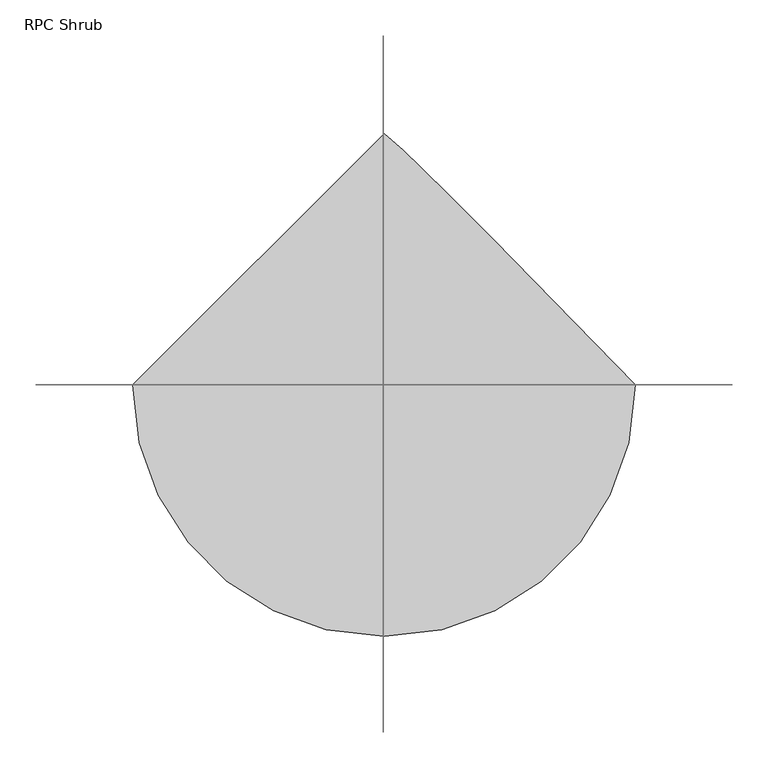
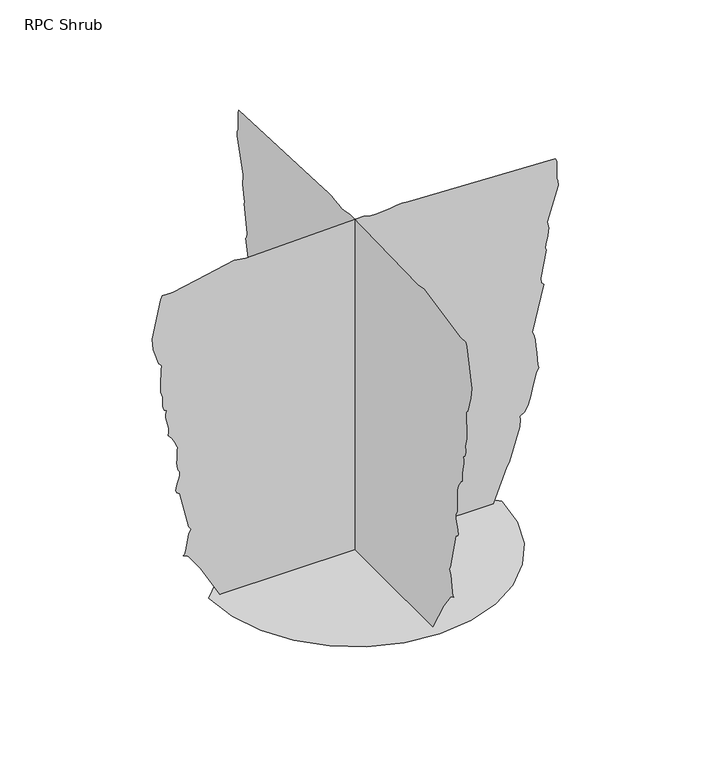
"""IFC4 building model written with IfcOpenShell, lengths in millimetres: geographic element geometry, RPC Shrub."""

from ifc_helpers import new_model, si_unit, origin, place, context, project, spatial, triangles, source, transform, mapped, element, save


def rpc_shrub_31a8b93a(model_context):
    return source(origin(), model_context, "Body", "Tessellation", [
        triangles([(-350.7919238, 0.0, 0.0), (-341.5167269, -80.3781425, 0.0), (-315.1055846, -154.1926595, 0.0), (-273.6723033, -219.3286546, 0.0), (-219.3286546, -273.6723033, 0.0), (-154.1926595, -315.1055846, 0.0), (-80.3781425, -341.5167269, 0.0), (1.53e-05, -350.7919238, 0.0), (80.3781425, -341.5167269, 0.0), (154.1926595, -315.1055846, 0.0), (219.3286546, -273.6723033, 0.0), (273.6723033, -219.3286546, 0.0), (315.1055846, -154.1926595, 0.0), (341.5167269, -80.3781425, 0.0), (350.7919238, 3.07e-05, 0.0), (236.7920327, 116.9354496, 0.0), (152.278414, 203.0298493, 0.0), (92.3366331, 263.4226928, 0.0), (52.0522189, 303.2555267, 0.0), (26.5109567, 327.6680809, 0.0), (10.7982689, 341.7996311, 0.0), (-4.6e-05, 350.7919238, 0.0), (-324.215748, 3.84e-05, 1.2173179), (-370.8406274, 3.35e-05, 83.4658628), (-399.9261703, 3.11e-05, 123.0734289), (-412.2293801, 3.08e-05, 129.051625), (-408.9211155, 3.06e-05, 131.6657641), (-406.1157635, 3.01e-05, 140.3154633), (-403.6090124, 2.93e-05, 152.586453), (-401.2018192, 2.85e-05, 166.0644457), (-398.6976843, 2.78e-05, 178.3356989), (-395.8897161, 2.73e-05, 186.9853889), (-392.5840676, 2.72e-05, 189.5995281), (-398.4933726, 2.67e-05, 197.4594953), (-420.6166225, 2.13e-05, 288.7310862), (-428.0425501, 2.09e-05, 294.8263719), (-430.4602441, 2.06e-05, 300.2222816), (-429.3784424, 2.01e-05, 307.9153985), (-426.2954184, 1.96e-05, 317.0255619), (-422.7147503, 1.9e-05, 326.6727201), (-420.1294066, 1.84e-05, 335.9714985), (-420.0429657, 1.8e-05, 344.0470593), (-423.9458525, 1.76e-05, 350.0113755), (-425.7846574, 1.73e-05, 354.1133054), (-426.7642851, 1.69e-05, 361.0677501), (-427.0864675, 1.64e-05, 370.0050679), (-426.9502839, 1.58e-05, 380.0529648), (-426.549509, 1.52e-05, 390.3444878), (-426.0858745, 1.46e-05, 400.0073791), (-425.7532276, 1.41e-05, 408.1745768), (-426.4709164, 1.4e-05, 410.2203094), (-428.5533111, 1.37e-05, 415.1395223), (-431.6808455, 1.33e-05, 421.8555731), (-435.5339533, 1.29e-05, 429.2946176), (-439.7930683, 1.24e-05, 436.3773974), (-444.1438565, 1.21e-05, 442.0247635), (-448.2641356, 1.19e-05, 445.1627987), (-446.5798634, 1.13e-05, 454.7627941), (-447.3237496, 1.08e-05, 464.614264), (-449.4533072, 1.02e-05, 474.4814306), (-451.9312446, 9.6e-06, 484.1285889), (-453.7228867, 9.1e-06, 493.3199973), (-453.7857462, 8.6e-06, 501.8172257), (-451.0825682, 8.1e-06, 509.3872215), (-457.0521166, 7.8e-06, 513.5415828), (-460.0617803, 7.5e-06, 518.8850793), (-461.0545249, 7.1e-06, 525.1768464), (-460.9785848, 6.8e-06, 532.1810337), (-460.7742731, 6.3e-06, 539.6645885), (-461.3898242, 5.8e-06, 547.3865009), (-463.7682037, 5.4e-06, 555.1136819), (-465.4157776, 5e-06, 561.3556337), (-466.1335027, 4.5e-06, 570.2405565), (-466.1439672, 3.8e-06, 581.0454929), (-465.6829488, 3.1e-06, 593.0448332), (-464.9731084, 2.4e-06, 605.510424), (-464.2449188, 1.7e-06, 617.7193445), (-463.7263095, 1e-06, 628.9433687), (-470.1830375, 6e-07, 635.4603401), (-483.6125957, -1.9e-06, 676.427389), (-486.0826484, -3.5e-06, 702.6813824), (-466.3063846, -9e-06, 796.8138634), (-462.2385006, -9.5e-06, 805.2351517), (-438.2030854, -9.5e-06, 803.62166), (-381.0850239, -1.02e-05, 816.2312828), (-289.6819184, -1.13e-05, 834.6638786), (-262.1915724, -1.1e-05, 829.9909081), (19.7347647, -1.14e-05, 837.0396057), (36.4753217, -1.12e-05, 832.8983614), (52.296608, -1.11e-05, 831.9030006), (67.462788, -1.12e-05, 832.9979193), (82.2389482, -1.13e-05, 835.1195921), (96.8883266, -1.14e-05, 837.2072554), (111.6762684, -1.15e-05, 838.2), (126.8665476, -1.14e-05, 837.0396057), (479.274888, -1.05e-05, 822.2375296), (482.0540425, -1.02e-05, 815.387875), (482.1352512, -7.6e-06, 772.1760504), (484.9144057, -7.1e-06, 765.3237797), (485.7264201, -6.5e-06, 753.5574921), (460.142989, -1.5e-06, 669.9522755), (461.5653222, -8e-07, 658.6313822), (463.0243175, -4e-07, 652.6251354), (462.3327899, 0.0, 644.1305231), (460.3499167, 7e-07, 634.1428333), (457.937455, 1.3e-06, 623.6548834), (455.9546182, 1.9e-06, 613.6645775), (455.2630906, 2.4e-06, 605.1699288), (456.7194697, 2.7e-06, 599.1636821), (444.0233697, 6.7e-06, 532.4063107), (445.7521523, 7.5e-06, 520.3676559), (451.4335642, 7.8e-06, 514.408572), (423.5503098, 1.45e-05, 402.0793093), (427.5579503, 1.49e-05, 394.7738686), (430.3816515, 1.57e-05, 381.6796097), (432.4011867, 1.67e-05, 365.0203794), (433.985901, 1.78e-05, 347.0279094), (435.512988, 1.88e-05, 329.9207414), (437.3570615, 1.96e-05, 315.9306796), (439.8925899, 2.01e-05, 307.2814982), (433.6244405, 2.08e-05, 296.3508428), (428.6607173, 2.18e-05, 279.4270756), (424.1580125, 2.3e-05, 259.2303796), (419.2676497, 2.42e-05, 238.4762867), (413.1461483, 2.54e-05, 219.8847435), (404.9449047, 2.62e-05, 206.1736254), (393.8151698, 2.66e-05, 200.0618437), (395.5911152, 2.71e-05, 190.3960819), (393.6789499, 2.81e-05, 173.5480006), (368.6246289, 3.29e-05, 92.4128639), (362.8777413, 3.35e-05, 83.2136162), (329.8526496, 3.84e-05, 1.0798268), (-1.4096743, -322.8065317, 1.2173152), (-1.4096743, -369.4314111, 83.4658628), (-1.4096743, -398.5143379, 123.0734289), (-1.4096743, -410.8201638, 129.051625), (-1.4096743, -407.5118992, 131.6657641), (-1.4096743, -404.7065472, 140.3154633), (-1.4096743, -402.1997961, 152.586453), (-1.4096743, -399.7926029, 166.0647001), (-1.4096743, -397.2858519, 178.3356989), (-1.4096743, -394.4804998, 186.9853889), (-1.4096743, -391.1722352, 189.5995281), (-1.4096743, -397.0841563, 197.4594953), (-1.4096743, -419.2074062, 288.7310862), (-1.4096743, -426.6333338, 294.8263719), (-1.4096743, -429.0483753, 300.2222816), (-1.4096743, -427.9665736, 307.9153985), (-1.4096743, -424.886202, 317.0255619), (-1.4096743, -421.3054976, 326.6727201), (-1.4096743, -418.7201903, 335.9714985), (-1.4096743, -418.6311333, 344.0470593), (-1.4096743, -422.5366362, 350.0113755), (-1.4096743, -424.3727886, 354.1133054), (-1.4096743, -425.3550688, 361.0677501), (-1.4096743, -425.6772511, 370.0050679), (-1.4096743, -425.5410313, 380.0529648), (-1.4096743, -425.1402926, 390.3444878), (-1.4096743, -424.6766582, 400.0073791), (-1.4096743, -424.343975, 408.1745768), (-1.4096743, -425.0617001, 410.2203094), (-1.4096743, -427.1440948, 415.1395223), (-1.4096743, -430.2716291, 421.8555731), (-1.4096743, -434.1221209, 429.2946176), (-1.4096743, -438.383852, 436.3773974), (-1.4096743, -442.7346039, 442.0247635), (-1.4096743, -446.8522668, 445.1627987), (-1.4096743, -445.170647, 454.7627941), (-1.4096743, -445.9145333, 464.614264), (-1.4096743, -448.0440908, 474.4814306), (-1.4096743, -450.5220283, 484.1285889), (-1.4096743, -452.3110542, 493.3199973), (-1.4096743, -452.3765299, 501.8198782), (-1.4096743, -449.6733519, 509.3872215), (-1.4096743, -455.6429003, 513.5415828), (-1.4096743, -458.652564, 518.8850793), (-1.4096743, -459.6453086, 525.1768464), (-1.4096743, -459.5693321, 532.1810337), (-1.4096743, -459.3650205, 539.6645885), (-1.4096743, -459.9805716, 547.3865009), (-1.4096743, -462.3589874, 555.1136819), (-1.4096743, -464.0065613, 561.3556337), (-1.4096743, -464.7216702, 570.2405565), (-1.4096743, -464.7347508, 581.0454929), (-1.4096743, -464.2711164, 593.0448332), (-1.4096743, -463.561276, 605.510424), (-1.4096743, -462.8330864, 617.7193445), (-1.4096743, -462.3144407, 628.9433687), (-1.4096743, -468.7738212, 635.4603401), (-1.4096743, -482.2033793, 676.427389), (-1.4096743, -484.6734321, 702.6813824), (-1.4096743, -464.8971683, 796.8138634), (-1.4096743, -460.829248, 805.2351517), (-1.4096743, -436.7938691, 803.62166), (-1.4096743, -379.6757712, 816.2312828), (-1.4096743, -288.2727021, 834.6638786), (-1.4096743, -260.7818293, 829.9909081), (-1.4096743, 21.1445124, 837.0396057), (-1.4096743, 37.884806, 832.8983614), (-1.4096743, 53.7063557, 831.9030006), (-1.4096743, 68.8725357, 832.9979193), (-1.4096743, 83.6486914, 835.1195921), (-1.4096743, 98.2980698, 837.2072554), (-1.4096743, 113.0860116, 838.2), (-1.4096743, 128.2762908, 837.0396057), (-1.4096743, 480.6841407, 822.2375296), (-1.4096743, 483.4632952, 815.387875), (-1.4096743, 483.5444675, 772.1760504), (-1.4096743, 486.323622, 765.3237797), (-1.4096743, 487.1356364, 753.5574921), (-1.4096743, 461.5522053, 669.9522755), (-1.4096743, 462.9771546, 658.6339983), (-1.4096743, 464.4335338, 652.6251354), (-1.4096743, 463.7420062, 644.1305231), (-1.4096743, 461.7591331, 634.1428333), (-1.4096743, 459.3467076, 623.6548834), (-1.4096743, 457.3664506, 613.6645775), (-1.4096743, 456.6723069, 605.1699288), (-1.4096743, 458.1313022, 599.1636821), (-1.4096743, 445.4352021, 532.4063107), (-1.4096743, 447.1639847, 520.3676559), (-1.4096743, 452.8453966, 514.408572), (-1.4096743, 424.9595261, 402.0793093), (-1.4096743, 428.9672029, 394.7738686), (-1.4096743, 431.7934839, 381.6796097), (-1.4096743, 433.810403, 365.0203794), (-1.4096743, 435.3951173, 347.0279094), (-1.4096743, 436.9222406, 329.9207414), (-1.4096743, 438.7662778, 315.9306796), (-1.4096743, 441.3018062, 307.2814982), (-1.4096743, 435.0336568, 296.3508428), (-1.4096743, 430.0699336, 279.4270756), (-1.4096743, 425.5672288, 259.2303796), (-1.4096743, 420.676866, 238.4762867), (-1.4096743, 414.5554009, 219.8847435), (-1.4096743, 406.354121, 206.1736254), (-1.4096743, 395.2243861, 200.0618437), (-1.4096743, 397.0003315, 190.3960819), (-1.4096743, 395.0882026, 173.5482549), (-1.4096743, 370.0338816, 92.4128639), (-1.4096743, 364.2869576, 83.2136162), (-1.4096743, 331.264482, 1.0798217)], [[21, 22, 1], [20, 21, 1], [19, 20, 1], [18, 19, 1], [17, 18, 1], [17, 1, 2], [17, 2, 3], [17, 3, 4], [16, 17, 4], [16, 4, 5], [16, 5, 6], [16, 6, 7], [16, 7, 8], [16, 8, 9], [16, 9, 10], [16, 10, 11], [16, 11, 12], [15, 16, 12], [14, 15, 12], [13, 14, 12], [25, 26, 27], [131, 132, 23], [82, 83, 84], [95, 96, 97], [95, 97, 98], [25, 27, 28], [56, 57, 58], [131, 23, 24], [130, 131, 24], [129, 130, 24], [128, 129, 24], [127, 128, 24], [95, 98, 99], [95, 99, 100], [95, 100, 101], [95, 101, 102], [127, 24, 25], [127, 25, 28], [127, 28, 29], [127, 29, 30], [127, 30, 31], [127, 31, 32], [127, 32, 33], [127, 33, 34], [127, 34, 35], [111, 112, 113], [95, 102, 103], [95, 103, 104], [95, 104, 105], [95, 105, 106], [95, 106, 107], [95, 107, 108], [119, 120, 121], [81, 82, 84], [95, 108, 109], [95, 109, 110], [94, 95, 110], [93, 94, 110], [92, 93, 110], [91, 92, 110], [91, 110, 111], [90, 91, 111], [90, 111, 113], [89, 90, 113], [126, 127, 35], [125, 126, 35], [124, 125, 35], [123, 124, 35], [122, 123, 35], [121, 122, 35], [119, 121, 35], [118, 119, 35], [117, 118, 35], [116, 117, 35], [115, 116, 35], [114, 115, 35], [113, 114, 35], [89, 113, 35], [88, 89, 35], [87, 88, 35], [87, 35, 36], [87, 36, 37], [81, 84, 85], [80, 81, 85], [79, 80, 85], [78, 79, 85], [78, 85, 86], [78, 86, 87], [77, 78, 87], [76, 77, 87], [75, 76, 87], [74, 75, 87], [73, 74, 87], [72, 73, 87], [71, 72, 87], [70, 71, 87], [69, 70, 87], [68, 69, 87], [67, 68, 87], [66, 67, 87], [65, 66, 87], [64, 65, 87], [55, 56, 58], [62, 63, 64], [62, 64, 87], [61, 62, 87], [60, 61, 87], [59, 60, 87], [58, 59, 87], [55, 58, 87], [54, 55, 87], [53, 54, 87], [52, 53, 87], [51, 52, 87], [50, 51, 87], [49, 50, 87], [48, 49, 87], [47, 48, 87], [46, 47, 87], [45, 46, 87], [44, 45, 87], [43, 44, 87], [42, 43, 87], [41, 42, 87], [37, 38, 39], [37, 39, 40], [87, 37, 40], [41, 87, 40], [135, 136, 137], [241, 242, 133], [192, 193, 194], [205, 206, 207], [205, 207, 208], [135, 137, 138], [166, 167, 168], [241, 133, 134], [240, 241, 134], [239, 240, 134], [238, 239, 134], [237, 238, 134], [205, 208, 209], [205, 209, 210], [205, 210, 211], [205, 211, 212], [237, 134, 135], [237, 135, 138], [237, 138, 139], [237, 139, 140], [237, 140, 141], [237, 141, 142], [237, 142, 143], [237, 143, 144], [237, 144, 145], [221, 222, 223], [205, 212, 213], [205, 213, 214], [205, 214, 215], [205, 215, 216], [205, 216, 217], [205, 217, 218], [229, 230, 231], [191, 192, 194], [205, 218, 219], [205, 219, 220], [204, 205, 220], [203, 204, 220], [202, 203, 220], [201, 202, 220], [201, 220, 221], [200, 201, 221], [200, 221, 223], [199, 200, 223], [236, 237, 145], [235, 236, 145], [234, 235, 145], [233, 234, 145], [232, 233, 145], [231, 232, 145], [229, 231, 145], [228, 229, 145], [227, 228, 145], [226, 227, 145], [225, 226, 145], [224, 225, 145], [223, 224, 145], [199, 223, 145], [198, 199, 145], [197, 198, 145], [197, 145, 146], [197, 146, 147], [191, 194, 195], [190, 191, 195], [189, 190, 195], [188, 189, 195], [188, 195, 196], [188, 196, 197], [187, 188, 197], [186, 187, 197], [185, 186, 197], [184, 185, 197], [183, 184, 197], [182, 183, 197], [181, 182, 197], [180, 181, 197], [179, 180, 197], [178, 179, 197], [177, 178, 197], [176, 177, 197], [175, 176, 197], [174, 175, 197], [165, 166, 168], [172, 173, 174], [172, 174, 197], [171, 172, 197], [170, 171, 197], [169, 170, 197], [168, 169, 197], [165, 168, 197], [164, 165, 197], [163, 164, 197], [162, 163, 197], [161, 162, 197], [160, 161, 197], [159, 160, 197], [158, 159, 197], [157, 158, 197], [156, 157, 197], [155, 156, 197], [154, 155, 197], [153, 154, 197], [152, 153, 197], [151, 152, 197], [147, 148, 149], [147, 149, 150], [197, 147, 150], [151, 197, 150]], closed=False),
    ])


if __name__ == "__main__":
    model = new_model("IFC4")
    model_context = context("Model", 3, world=origin())
    ifc_project = project(units=[si_unit("LENGTHUNIT", "METRE", prefix="MILLI")], contexts=[model_context])
    site = spatial("IfcSite", under=ifc_project)
    building = spatial("IfcBuilding", under=site)
    placement = place(None, origin())
    rpc_shrub_shape = rpc_shrub_31a8b93a(model_context)
    element("IfcGeographicElement", 1, ObjectType="RPC Shrub", at=placement, inside=building, context=model_context, shape_type="MappedRepresentation", body=[
        mapped(rpc_shrub_shape, transform((0.0, 0.0, 0.0), x_axis=(1.0, 0.0, 0.0), y_axis=(0.0, 1.0, 0.0), z_axis=(0.0, 0.0, 1.0))),
    ])
    save(model, "model.ifc")

# Revit data of these elements
# Type "RPC Shrub"
#   Type Comments = "Boxwood"
#   built-in parameter 1005198 = "{2, 15},{39, RPC-16-G0M3-8AG0-UBW3-U000-ST1L-LVER-AU},{1, 0},{1, 0},{2, 13},{1, 8},{5, Color},{1, 0},{1, 0},{3, 0.8},{3, 0.8},{3, 0.8},{1, 8},{7, BBoxMin},{1, 0},{1, 0},{1, 0},{1, 0},{1, 0},{1, 8},{7, BBoxMax},{1, 0},{1, 0},{1, 0},{1, 0},{1, 0},{2, 11},{9, RPCTypeId},{1, 0},{1, 0},{39, RPC-16-G0M3-8AG0-UBW3-U000-ST1L-LVER-AU},{1, 6},{14, RPCPlantHeight},{1, 0},{1, 0},{4, 2.75},{2, 11},{7, keyword},{1, 0},{1, 0},{35, :RPCs:Shrubs & Grasses:Geometry:RPC},{2, 11},{8, category},{1, 0},{1, 0},{16, Shrubs & Grasses},{2, 11},{12, LocalizedUID},{1, 0},{1, 0},{7, Boxwood},{2, 14},{6, Height},{1, 0},{1, 0},{4, 2.75},{1, 2},{16, Cast Reflections},{1, 0},{1, 0},{1, 0},{1, 2},{12, Cast Shadows},{1, 0},{1, 0},{1, 1},{1, 2},{9, Lock View},{1, 0},{1, 0},{1, 0},{1, 4},{5, ViewC},{1, 0},{1, 0},{1, 0},{21, assetlibrary_base.fbx},{1, 5},"
#   built-in parameter 1005195 = "RPC-16-G0M3-8AG0-UBW3-U000-ST1L-LVER-AU"
#   Assembly Code = "G2050500"
#   Height = 2' - 9"
#   Default Elevation = 0
